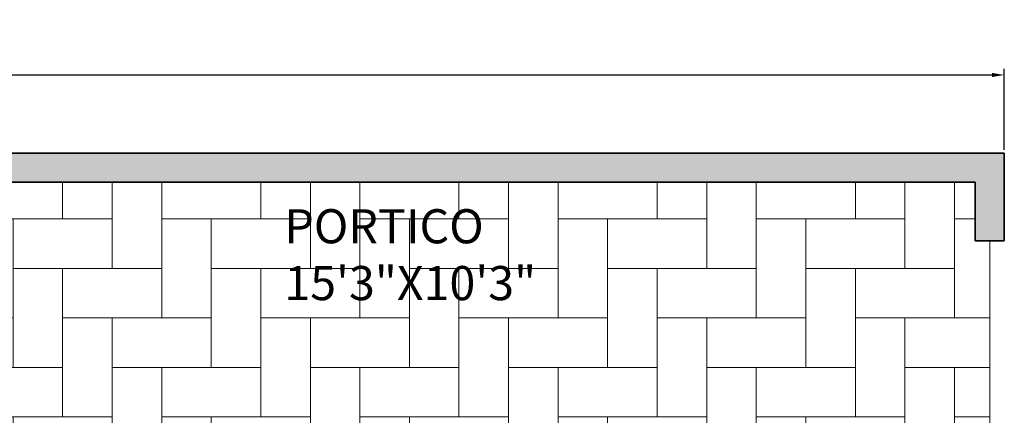
# Model space of a CAD drawing. Units: inches. Extents: x 2337 to 3570, y 1258 to 1938.
# Tile 19 of 30: x 2704 to 2906, y 1839 to 1920. Entities that reach past the tile are written whole.
import ezdxf

# ---------------------------------------------------------------- set-up
doc = ezdxf.new("R2010")
doc.units = ezdxf.units.IN
for name, color, linetype, lineweight in [('A-ANNO-DIMS', 2, 'Continuous', 18), ('A-AREA-IDEN', 7, 'Continuous', 18), ('A-FLOR-PATT', 252, 'Continuous', 13), ('C-PROP', 7, 'Continuous', 35), ('L-SITE-GATE', 4, 'Continuous', 18)]:
    doc.layers.add(name, color=color, linetype=linetype, lineweight=lineweight)
doc.layers.add('C-PROP-PATT', color=251, linetype='Continuous', lineweight=13, true_color=0x636466)
doc.styles.get("Standard").update_dxf_attribs({"font": 'arial.ttf'})
doc.dimstyles.new('ISO-25', dxfattribs={"dimtxt": 9, "dimasz": 2.5, "dimexe": 1.25, "dimexo": 0.625, "dimtad": 1, "dimdec": 1, "dimlunit": 3, "dimtxsty": 'Standard', "dimcen": 2.5, "dimadec": 0, "dimazin": 0, "dimtfac": 1, "dimtdec": 1, "dimtmove": 0, "dimatfit": 3, "dimfxl": 1, "dimarcsym": 0})

# ---------------------------------------------------------------- blocks, each defined once
blk = doc.blocks.new('*D6')
at = {"layer": 'A-ANNO-DIMS', "color": 0, "lineweight": -2, "transparency": 16777216}
for p, q in [((2425.84, 1893.74), (2425.84, 1910.39)), ((2905.84, 1893.74), (2905.84, 1910.39)), ((2428.34, 1909.14), (2903.34, 1909.14))]:
    blk.add_line(p, q, dxfattribs=at)
at = {"layer": 'A-ANNO-DIMS', "color": 0, "transparency": 16777216}
for points in [[(2428.34, 1909.55), (2428.34, 1908.72), (2425.84, 1909.14)], [(2903.34, 1909.55), (2903.34, 1908.72), (2905.84, 1909.14)]]:
    blk.add_solid(points, dxfattribs=at)
at = {"layer": 'Defpoints', "color": 0, "transparency": 16777216}
for p in [(2905.84, 1909.14), (2425.84, 1893.12), (2905.84, 1893.12)]:
    blk.add_point(p, dxfattribs=at)
at = {"layer": 'A-ANNO-DIMS', "color": 0, "transparency": 16777216, "insert": (2665.84, 1914.36), "char_height": 9, "attachment_point": 5}
blk.add_mtext("40'", dxfattribs=at)

msp = doc.modelspace()

# ---------------------------------------------------------------- hatches: boundary and pattern name
at = {"layer": 'A-FLOR-PATT', "transparency": 33554687}
h = msp.add_hatch(dxfattribs=at)
h.set_pattern_fill('AR-HBONE', color=256, scale=0.1, angle=45)
h.paths.add_polyline_path([(2902.84, 1875.12), (2899.84, 1875.12), (2899.84, 1887.12), (2671.84, 1887.12), (2671.84, 1857.12), (2681.84, 1857.12), (2681.84, 1810.12), (2719.84, 1810.12), (2719.84, 1764.12), (2872.84, 1764.12), (2899.84, 1764.12), (2899.84, 1779.12), (2902.84, 1779.12)])
h.paths.add_polyline_path([(2854.18, 1832.56), (2857.32, 1832.42), (2861.94, 1831.21, -0.088302), (2868.63, 1828.11), (2871.77, 1825.92, -0.105467), (2873.27, 1824.31), (2874.97, 1823.99), (2877.34, 1822.55), (2875.42, 1827.3), (2873.36, 1826.95, -0.132795), (2873.22, 1833.51), (2876.1, 1833.32), (2876.1, 1832.97), (2877.28, 1832.48, -0.091085), (2878.86, 1831.44, -0.069602), (2881.45, 1828.18, -0.141553), (2886.25, 1809.41, -0.141553), (2881.49, 1790.63, -0.069602), (2878.91, 1787.37, -0.091085), (2877.32, 1786.33), (2876.14, 1785.83, -0.354729), (2875.73, 1785.45), (2873.27, 1785.29, -0.132795), (2873.39, 1791.84), (2875.45, 1791.49), (2877.36, 1796.25), (2874.99, 1794.81), (2873.3, 1794.48, -0.105467), (2871.8, 1792.87), (2868.67, 1790.67, -0.088302), (2861.99, 1787.56), (2857.37, 1786.34), (2854.23, 1786.2), (2827.8, 1783.01, -0.315912), (2819.63, 1782.95), (2793.54, 1785.74), (2798.79, 1786.94), (2825.85, 1785.28, 0.026512), (2832.53, 1785.23), (2857.37, 1786.34), (2861.99, 1787.56, 0.088302), (2868.67, 1790.67), (2871.8, 1792.87, 0.191215), (2873.93, 1796.11), (2875.79, 1805.13, 0.102572), (2875.78, 1813.67), (2873.91, 1822.68, 0.191215), (2871.77, 1825.92), (2868.63, 1828.11, 0.088302), (2861.94, 1831.21), (2857.32, 1832.42), (2832.48, 1833.49, 0.026512), (2825.8, 1833.42), (2798.75, 1831.7), (2793.5, 1832.9), (2819.58, 1835.73, -0.315912), (2827.75, 1835.69)], flags=16)
h.paths.add_polyline_path([(2862.34, 1826.57), (2867.3, 1826, -0.316515), (2870.31, 1823.31), (2872.44, 1814.15, -0.11452), (2872.45, 1804.64), (2870.34, 1795.48, -0.316515), (2867.33, 1792.79), (2862.37, 1792.2, -0.464922), (2861.4, 1793.12), (2861.86, 1801.97), (2861.84, 1809.39), (2861.85, 1816.81), (2861.36, 1825.65, -0.464922)], flags=16)
h.paths.add_polyline_path([(2821.29, 1791.09), (2807.57, 1791.5, -0.405226), (2805.02, 1794.12), (2805.02, 1794.12, 0.40508), (2807.57, 1791.5), (2821.29, 1791.09, 0.423258), (2824, 1793.72), (2824, 1793.72, -0.423258)], flags=16)
h.paths.add_polyline_path([(2879.43, 1814.8), (2881.74, 1813.82), (2882.58, 1811.67), (2882.72, 1809.41), (2882.59, 1807.14), (2881.75, 1804.99), (2879.44, 1804.01), (2880.04, 1807.7, 0.081616), (2880.04, 1811.11)], flags=0)
h.paths.add_polyline_path([(2796.96, 1829.72), (2796.14, 1815.43, 0.029076), (2796.15, 1803.21), (2797, 1788.93, -0.409057), (2796.19, 1788), (2791.05, 1787.61), (2785.76, 1792.94, -0.173254), (2784.26, 1796.14), (2783.47, 1804.33, -0.047466), (2783.46, 1814.29), (2784.23, 1822.48, -0.173254), (2785.73, 1825.69), (2791.01, 1831.02), (2796.15, 1830.64, -0.409057)], flags=16)
h.paths.add_polyline_path([(2750.34, 1835.79), (2750.01, 1834.37, 0.040009), (2748.77, 1826.06), (2748.63, 1824.02), (2750.53, 1825.24), (2756.61, 1827.24), (2771.95, 1829.42), (2781.4, 1831.05), (2780.1, 1822.89), (2779.44, 1814.33), (2779.14, 1809.3), (2779.45, 1804.28), (2780.13, 1795.72), (2781.44, 1787.56), (2771.99, 1789.17), (2756.65, 1791.34), (2750.56, 1793.32), (2748.66, 1794.54), (2748.8, 1792.49, 0.040009), (2750.06, 1784.19), (2750.4, 1782.77), (2745.9, 1784.64), (2744.1, 1788.13), (2743.1, 1791.92), (2741.07, 1803), (2740.86, 1809.27), (2741.06, 1815.55), (2743.06, 1826.62), (2744.06, 1830.42), (2745.85, 1833.91)], flags=16)
h.paths.add_polyline_path([(2761.18, 1831.2), (2754.85, 1829.51), (2754.56, 1830.83, -0.143032), (2754.62, 1831.81), (2755.05, 1833), (2761.17, 1831.71, -0.789416)], flags=16)
h.paths.add_polyline_path([(2761.23, 1787.38), (2754.89, 1789.06), (2754.6, 1787.74, 0.143032), (2754.66, 1786.76), (2755.1, 1785.57), (2761.21, 1786.87, 0.789416)], flags=16)
h.paths.add_polyline_path([(2689.03, 1816.17), (2701.27, 1816.17), (2701.27, 1823.8), (2689.03, 1823.8)], flags=24)
h.paths.add_polyline_path([(2755.38, 1858.95), (2808.72, 1858.95), (2808.72, 1885.07), (2755.38, 1885.07)], flags=24)
at = {"layer": 'C-PROP-PATT'}
h = msp.add_hatch(color=256, dxfattribs=at)
h.dxf.hatch_style = 1
h.paths.add_polyline_path([(2905.84, 1893.12), (2425.84, 1893.12), (2425.84, 1293.12), (2731.84, 1293.12), (2731.84, 1299.12), (2431.84, 1299.12), (2431.84, 1887.12), (2899.84, 1887.12), (2899.84, 1875.12), (2905.84, 1875.12)])
h.paths.add_polyline_path([(2845.84, 1299.12), (2827.84, 1299.12), (2827.84, 1293.12), (2845.84, 1293.12)], flags=17)
h.paths.add_polyline_path([(2905.84, 1779.12), (2899.84, 1779.12), (2899.84, 1299.12), (2893.84, 1299.12), (2893.84, 1293.12), (2905.84, 1293.12)], flags=17)

# ---------------------------------------------------------------- linework, layer by layer
at = {"layer": 'C-PROP'}
for p, q in [((2425.84, 1893.12), (2905.84, 1893.12)), ((2905.84, 1893.12), (2905.84, 1875.12)), ((2431.84, 1887.12), (2899.84, 1887.12)), ((2899.84, 1887.12), (2899.84, 1875.12)), ((2899.84, 1875.12), (2905.84, 1875.12))]:
    msp.add_line(p, q, dxfattribs=at)
at = {"layer": 'L-SITE-GATE'}
msp.add_line((2902.84, 1875.12), (2902.84, 1779.12), dxfattribs=at)

# ---------------------------------------------------------------- texts
at = {"layer": 'A-AREA-IDEN', "insert": (2758.2, 1881.59), "char_height": 7, "attachment_point": 1}
msp.add_mtext_dynamic_manual_height_columns('PORTICO\\P15\'3"X10\'3"', width=66.911, gutter_width=12.5, heights=[0], dxfattribs=at)

# ---------------------------------------------------------------- dimensions: what is measured, and where the dimension line sits
at = {"layer": 'A-ANNO-DIMS'}
dim = msp.add_linear_dim(base=(2905.84, 1909.14), p1=(2425.84, 1893.12), p2=(2905.84, 1893.12), dimstyle='ISO-25', override={"dimclrd": 0, "dimclre": 0, "dimclrt": 0}, dxfattribs=at)
dim.commit()
dim.dimension.update_dxf_attribs({"geometry": '*D6', "text_midpoint": (2665.84, 1914.36)})

doc.saveas('drawing.dxf')
